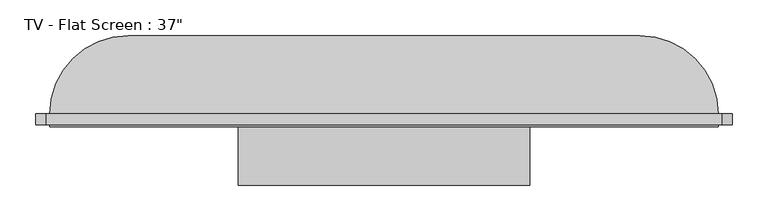
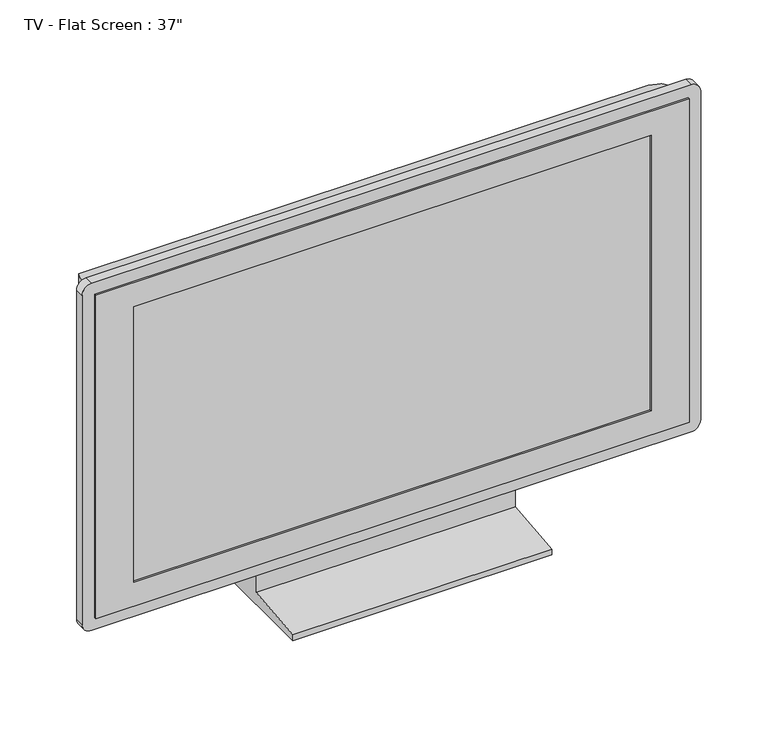
"""IFC4 building model written with IfcOpenShell, lengths in millimetres: furniture geometry."""

from ifc_helpers import new_model, si_unit, point, frame, frame_2d, origin, place, context, project, spatial, polyline, circle_curve, ellipse_curve, trimmed, segment, composite_curve, outline, extrude, faceted_brep, source, transform, mapped, element, save
from ifc_brep_helpers import plane_surface, cylinder_surface, advanced_brep


def furniture_4831bac8(model_context):
    return source(origin(), model_context, "Body", "SolidModel", [
        extrude(outline(polyline([(-51.4613764, 80.0), (-1.4613764, 80.0), (48.5386236, 0.0), (-151.4613764, 0.0), (-151.4613764, 10.0), (-51.4613764, 20.0), (-51.4613764, 80.0)])), frame((-208.760248, 0.0, 0.0), z_axis=(1.0, 0.0, 0.0), x_axis=(0.0, 1.0, 0.0)), (0.0, 0.0, 1.0), 409.6314677),
        faceted_brep([(465.6869536, -69.4613764, 620.8776873), (-473.5759818, -69.4613764, 620.8776873), (-473.5759818, -69.4613764, 80.0), (465.6869536, -69.4613764, 80.0), (-413.5759818, -69.4613764, 580.8776873), (405.6869536, -69.4613764, 580.8776873), (405.6869536, -69.4613764, 120.0), (-413.5759818, -69.4613764, 120.0), (465.6869536, -51.4613764, 620.8776873), (465.6869536, -51.4613764, 80.0), (-473.5759818, -51.4613764, 80.0), (-473.5759818, -51.4613764, 620.8776873), (-413.5759818, -66.4613764, 580.8776873), (-413.5759818, -66.4613764, 120.0), (405.6869536, -66.4613764, 120.0), (405.6869536, -66.4613764, 580.8776873)], [[[0, 1, 2, 3], [4, 5, 6, 7]], [[8, 9, 10, 11]], [[1, 0, 8, 11]], [[2, 1, 11, 10]], [[3, 2, 10, 9]], [[0, 3, 9, 8]], [[12, 13, 14, 15]], [[12, 15, 5, 4]], [[15, 14, 6, 5]], [[14, 13, 7, 6]], [[13, 12, 4, 7]]]),
        extrude(outline(composite_curve([segment(polyline([(640.8776873, 470.6869536), (640.8776873, -478.5759818)]), True, "CONTINUOUS"), segment(trimmed(circle_curve(frame_2d((625.8776873, -478.5759818)), 15.0), [point((640.8776873, -478.5759818))], [point((625.8776873, -493.5759818))], False, "CARTESIAN"), True, "CONTINUOUS"), segment(polyline([(625.8776873, -493.5759818), (75.0, -493.5759818)]), True, "CONTINUOUS"), segment(trimmed(circle_curve(frame_2d((75.0, -478.5759818)), 15.0), [point((75.0, -493.5759818))], [point((60.0, -478.5759818))], False, "CARTESIAN"), True, "CONTINUOUS"), segment(polyline([(60.0, -478.5759818), (60.0, 470.6869536)]), True, "CONTINUOUS"), segment(trimmed(circle_curve(frame_2d((75.0, 470.6869536)), 15.0), [point((60.0, 470.6869536))], [point((75.0, 485.6869536))], False, "CARTESIAN"), True, "CONTINUOUS"), segment(polyline([(75.0, 485.6869536), (625.8776873, 485.6869536)]), True, "CONTINUOUS"), segment(trimmed(circle_curve(frame_2d((625.8776873, 470.6869536)), 15.0), [point((625.8776873, 485.6869536))], [point((640.8776873, 470.6869536))], False, "CARTESIAN"), True, "CONTINUOUS")], self_intersect=False), holes=[polyline([(620.8776873, 465.6869536), (80.0, 465.6869536), (80.0, -473.5759818), (620.8776873, -473.5759818), (620.8776873, 465.6869536)])]), frame((0.0, -66.4613764, 0.0), z_axis=(0.0, 1.0, 0.0), x_axis=(0.0, 0.0, 1.0)), (0.0, 0.0, 1.0), 15.0),
        advanced_brep(
        [(-473.5759818, -51.4613764, 80.0), (465.6869536, -51.4613764, 80.0), (465.6869536, -51.4613764, 620.8776873), (-473.5759818, -51.4613764, 620.8776873), (355.6869536, 58.5386236, 80.0), (-363.5759818, 58.5386236, 80.0), (-363.5759818, 58.5386236, 510.8776873), (355.6869536, 58.5386236, 510.8776873)],
        [
            (0, 1),
            (1, 2),
            (2, 3),
            (3, 0),
            (4, 5),
            (5, 6),
            (6, 7),
            (7, 4),
            (0, 5, circle_curve(frame((-363.5759818, -51.4613764, 80.0), z_axis=(0.0, 0.0, -1.0), x_axis=(-1.0, 0.0, 0.0)), 110.0)),
            (4, 1, circle_curve(frame((355.6869536, -51.4613764, 80.0), z_axis=(0.0, 0.0, -1.0), x_axis=(1.0, 0.0, 0.0)), 110.0)),
            (7, 2, ellipse_curve(frame((355.6869536, -51.4613764, 510.8776873), z_axis=(0.7071067811865475, 0.0, -0.7071067811865475), x_axis=(0.7071067811865474, 0.0, 0.7071067811865476)), 155.5634919, 110.0)),
            (6, 3, ellipse_curve(frame((-363.5759818, -51.4613764, 510.8776873), z_axis=(0.7071067811865475, 0.0, 0.7071067811865475), x_axis=(-0.7071067811865476, 0.0, 0.7071067811865474)), 155.5634919, 110.0)),
        ],
        [
            plane_surface(frame((-473.5759818, -51.4613764, 620.8776873), z_axis=(0.0, -1.0, 0.0), x_axis=(-1.0, 0.0, 0.0))),
            plane_surface(frame((-473.5759818, 58.5386236, 620.8776873), z_axis=(0.0, 1.0, 0.0), x_axis=(1.0, 0.0, 0.0))),
            plane_surface(frame((-473.5759818, -51.4613764, 80.0), z_axis=(0.0, 0.0, -1.0), x_axis=(0.0, 1.0, 0.0))),
            cylinder_surface(frame((355.6869536, -51.4613764, 80.0), z_axis=(0.0, 0.0, 1.0), x_axis=(1.0, 0.0, 0.0)), 110.0),
            cylinder_surface(frame((465.6869536, -51.4613764, 510.8776873), z_axis=(-1.0, 0.0, 0.0), x_axis=(0.0, 0.0, 1.0)), 110.0),
            cylinder_surface(frame((-363.5759818, -51.4613764, 620.8776873), z_axis=(0.0, 0.0, -1.0), x_axis=(-1.0, 0.0, 0.0)), 110.0),
        ],
        [
            (0, [[1, 2, 3, 4]]),
            (1, [[5, 6, 7, 8]]),
            (2, [[-1, 9, -5, 10]]),
            (3, [[11, -2, -10, -8]]),
            (4, [[-11, -7, 12, -3]]),
            (5, [[-12, -6, -9, -4]]),
        ],
    ),
    ])


if __name__ == "__main__":
    model = new_model("IFC4")
    model_context = context("Model", 3, world=origin())
    ifc_project = project(units=[si_unit("LENGTHUNIT", "METRE", prefix="MILLI")], contexts=[model_context])
    site = spatial("IfcSite", under=ifc_project)
    building = spatial("IfcBuilding", under=site)
    placement = place(None, origin())
    furniture_shape = furniture_4831bac8(model_context)
    element("IfcFurniture", 1, ObjectType="TV - Flat Screen : 37\"", at=placement, inside=building, context=model_context, shape_type="MappedRepresentation", body=[
        mapped(furniture_shape, transform((0.0, 0.0, 0.0), x_axis=(1.0, 0.0, 0.0), y_axis=(0.0, 1.0, 0.0), z_axis=(0.0, 0.0, 1.0))),
    ])
    save(model, "model.ifc")

# Revit data of these elements
# Type "TV - Flat Screen : 37\""
#   SinAng = 0' - 0.0193"
#   L = 2' - 8.25445"
#   H = 1' - 6.14479"
#   Thickness = 0' - 4.33071"
#   Diagonal = 3' - 1.00787"
#   CosAng = 0' - 0.03431"
#   Stand [instance default] = yes
#   Default Elevation = 0
# Element 1 (IfcFurniture, "TV - Flat Screen : 37\"")
#   Materials on its faces: "TV - Black", "TV - Glass", "TV - Screen"
# Materials
#   "TV - Black": colour RGB 49 49 49, transparency 0
#   "TV - Glass": colour RGB 157 157 157, transparency 0.9
#   "TV - Screen": colour RGB 0 0 0, transparency 0
